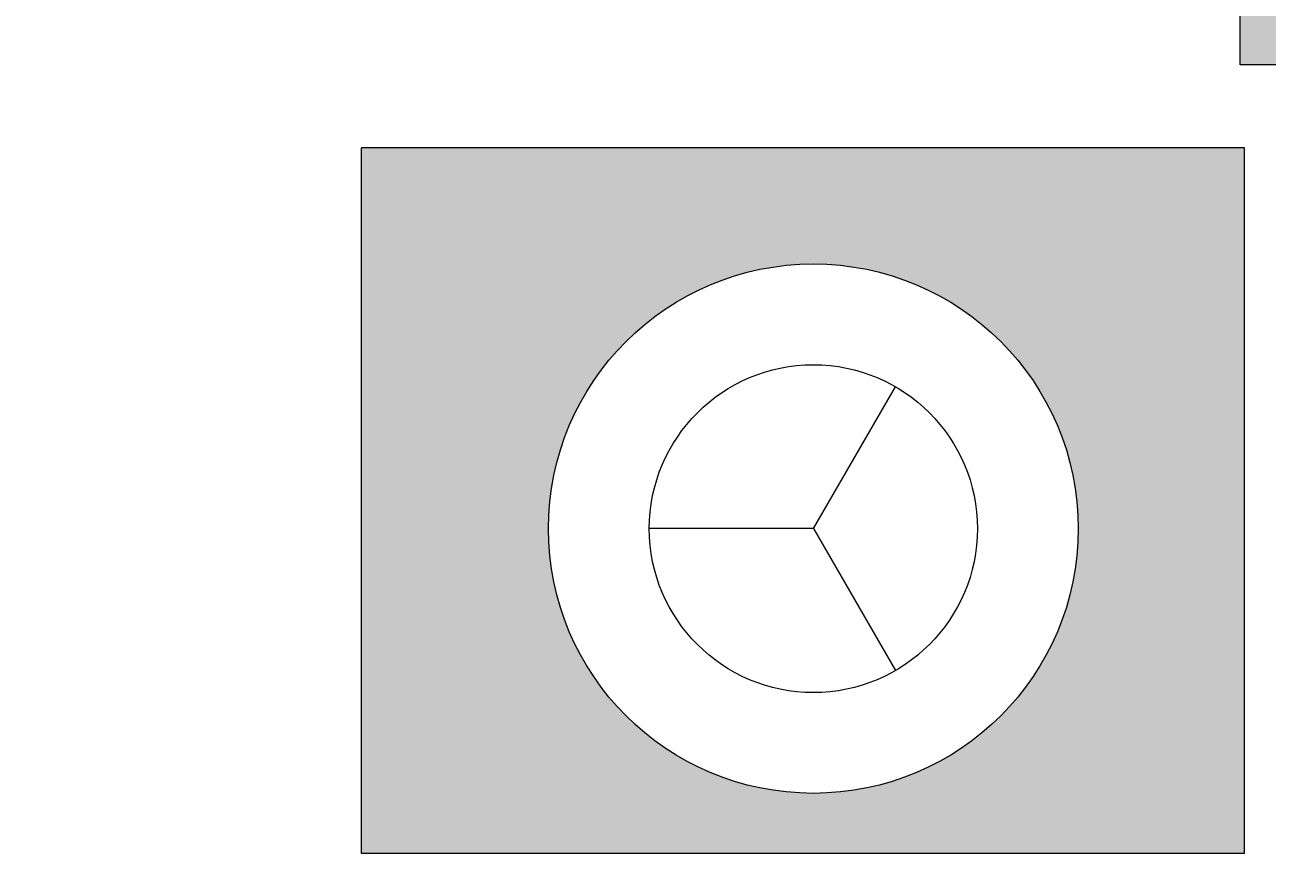
# Model space of a CAD drawing. Units: millimetres. Extents: x 27017497 to 27018854, y 7058029 to 7059154.
# Tile 20 of 91: x 27017651 to 27017679, y 7058144 to 7058163. Entities that reach past the tile are written whole.
import ezdxf

# ---------------------------------------------------------------- set-up
doc = ezdxf.new("R2010")
doc.units = ezdxf.units.MM
doc.layers.add('A-ANNO-DIMS', color=2, linetype='Continuous', lineweight=18)
doc.layers.add('A-FURN', color=8, linetype='Continuous', lineweight=18)
doc.layers.add('A-FURN-PATT', color=177, linetype='Continuous', lineweight=13, true_color=0x293189)
doc.styles.get("Standard").update_dxf_attribs({"font": 'arial.ttf'})
doc.dimstyles.get("Standard").update_dxf_attribs({"dimtxt": 0.18, "dimasz": 0.18, "dimexe": 0.18, "dimexo": 0.0625, "dimgap": 0.09, "dimtad": 0, "dimtih": 1, "dimtoh": 1, "dimdec": 4, "dimzin": 0, "dimdsep": 46, "dimtxsty": 'Standard', "dimcen": 0.09, "dimadec": 0, "dimazin": 0, "dimtfac": 1, "dimtdec": 4, "dimtofl": 0, "dimtmove": 0, "dimatfit": 3, "dimfxl": 1, "dimtolj": 1, "dimtzin": 0, "dimarcsym": 0})

# ---------------------------------------------------------------- blocks, each defined once
blk = doc.blocks.new('CAMMAT')
for p, q in [((0.68, -0.07), (0.68, -0.47)), ((0.68, -0.07), (1.18, -0.07)), ((1.18, -0.07), (1.18, -0.47)), ((0.92416, -0.2541), (0.87771, -0.17366)), ((0.92416, -0.2541), (0.87771, -0.33455)), ((0.92416, -0.2541), (1.01705, -0.2541)), ((0.68, -0.47), (1.18, -0.47)), ((-0.6904, -0.51693), (0.68256, -0.51693)), ((0.68256, -0.51693), (0.68256, -0.76028))]:
    blk.add_line(p, q)
for radius in [0.15, 0.09289]:
    blk.add_circle((0.92416, -0.2541), radius)
blk = doc.blocks.new('*D47')
at = {"layer": 'A-ANNO-DIMS', "color": 0, "lineweight": -2, "transparency": 16777216}
for p, q in [((27017561.166, 7058294.35), (27017561.166, 7058028.6)), ((27018790.606, 7058294.35), (27018790.606, 7058028.6)), ((27017561.346, 7058028.78), (27018175.431, 7058028.78)), ((27018790.426, 7058028.78), (27018176.341, 7058028.78))]:
    blk.add_line(p, q, dxfattribs=at)
at = {"layer": 'A-ANNO-DIMS', "color": 0, "transparency": 16777216}
for points in [[(27017561.346, 7058028.81), (27017561.346, 7058028.75), (27017561.166, 7058028.78)], [(27018790.426, 7058028.81), (27018790.426, 7058028.75), (27018790.606, 7058028.78)]]:
    blk.add_solid(points, dxfattribs=at)
at = {"layer": 'Defpoints', "color": 0, "transparency": 16777216}
for p in [(27017561.166, 7058294.412), (27018790.606, 7058294.412), (27018790.606, 7058028.78)]:
    blk.add_point(p, dxfattribs=at)
at = {"layer": 'A-ANNO-DIMS', "color": 0, "transparency": 16777216, "insert": (27018175.886, 7058028.78), "char_height": 0.18, "attachment_point": 5}
blk.add_mtext('\\A1;1229.4', dxfattribs=at)
blk = doc.blocks.new('*D48')
at = {"layer": 'A-ANNO-DIMS', "color": 0, "lineweight": -2, "transparency": 16777216}
for p, q in [((27018463.498, 7058622.912), (27017497.536, 7058622.912)), ((27017497.716, 7058622.732), (27017497.716, 7058357.753)), ((27017497.716, 7058092.41), (27017497.716, 7058357.389)), ((27018555.129, 7058092.23), (27017497.536, 7058092.23))]:
    blk.add_line(p, q, dxfattribs=at)
at = {"layer": 'A-ANNO-DIMS', "color": 0, "transparency": 16777216}
for points in [[(27017497.686, 7058622.732), (27017497.746, 7058622.732), (27017497.716, 7058622.912)], [(27017497.686, 7058092.41), (27017497.746, 7058092.41), (27017497.716, 7058092.23)]]:
    blk.add_solid(points, dxfattribs=at)
at = {"layer": 'Defpoints', "color": 0, "transparency": 16777216}
for p in [(27018463.561, 7058622.912), (27017497.716, 7058092.23), (27018555.192, 7058092.23)]:
    blk.add_point(p, dxfattribs=at)
at = {"layer": 'A-ANNO-DIMS', "color": 0, "transparency": 16777216, "insert": (27017497.716, 7058357.571), "char_height": 0.18, "attachment_point": 5}
blk.add_mtext('\\A1;530.7', dxfattribs=at)

msp = doc.modelspace()

# ---------------------------------------------------------------- hatches: boundary and pattern name
at = {"layer": 'A-FURN-PATT'}
h = msp.add_hatch(color=256, dxfattribs=at)
h.dxf.hatch_style = 1
h.paths.add_polyline_path([(27017731.53, 7058218.852, 0.414214), (27017729.937, 7058220.445), (27017681.344, 7058220.445, 0.414214), (27017679.751, 7058218.852), (27017679.751, 7058174.658), (27017683.647, 7058174.959), (27017687.23, 7058175.46), (27017689.748, 7058176.196), (27017691.461, 7058177.277), (27017692.628, 7058178.816), (27017693.508, 7058180.922), (27017694.36, 7058183.707), (27017694.963, 7058180.902), (27017695.506, 7058178.662), (27017696.096, 7058176.759), (27017696.84, 7058174.966), (27017697.847, 7058173.059), (27017699.222, 7058170.809), (27017701.073, 7058167.99), (27017703.508, 7058164.376), (27017705.943, 7058167.99), (27017707.794, 7058170.809), (27017709.169, 7058173.059), (27017710.176, 7058174.966), (27017710.92, 7058176.759), (27017711.51, 7058178.662), (27017712.053, 7058180.902), (27017712.656, 7058183.707), (27017713.508, 7058180.922), (27017714.388, 7058178.816), (27017715.555, 7058177.277), (27017717.268, 7058176.196), (27017719.786, 7058175.46), (27017723.369, 7058174.959), (27017728.274, 7058174.58), (27017731.53, 7058174.396)])
h.paths.add_polyline_path([(27017723.369, 7058174.959), (27017719.786, 7058175.46), (27017717.268, 7058176.196), (27017715.555, 7058177.277), (27017714.388, 7058178.816), (27017713.508, 7058180.922), (27017712.656, 7058183.707), (27017712.053, 7058180.902), (27017711.51, 7058178.662), (27017710.92, 7058176.759), (27017710.176, 7058174.966), (27017709.169, 7058173.059), (27017707.794, 7058170.809), (27017705.943, 7058167.99), (27017703.508, 7058164.376), (27017734.763, 7058174.214), (27017728.274, 7058174.58)])
h.paths.add_polyline_path([(27017696.84, 7058174.966), (27017696.096, 7058176.759), (27017695.506, 7058178.662), (27017694.963, 7058180.902), (27017694.36, 7058183.707), (27017693.508, 7058180.922), (27017692.628, 7058178.816), (27017691.461, 7058177.277), (27017689.748, 7058176.196), (27017687.23, 7058175.46), (27017683.647, 7058174.959), (27017679.751, 7058174.658), (27017678.741, 7058174.58), (27017672.253, 7058174.214), (27017703.508, 7058164.376), (27017701.073, 7058167.99), (27017699.222, 7058170.809), (27017697.847, 7058173.059)])
h.paths.add_polyline_path([(27017678.454, 7058172.262), (27017678.454, 7058162.569), (27017733.139, 7058162.569), (27017733.139, 7058173.703), (27017703.508, 7058164.376)])
h.paths.add_polyline_path([(27017730.145, 7058158.291, 0.41419), (27017728.95, 7058159.485), (27017707.491, 7058159.485, 0.414214), (27017706.296, 7058158.29), (27017706.296, 7058148.731, 0.414214), (27017707.491, 7058147.536), (27017728.95, 7058147.536, 0.414237), (27017730.145, 7058148.731)], flags=0)
h.paths.add_polyline_path([(27017731.53, 7058162.569), (27017679.751, 7058162.569), (27017679.751, 7058146.361, 0.414214), (27017681.344, 7058144.768), (27017729.937, 7058144.768, 0.414214), (27017731.53, 7058146.361)])
h.paths.add_polyline_path([(27017703.354, 7058159.485, -0.41419), (27017704.549, 7058158.291), (27017704.549, 7058148.731, -0.414237), (27017703.354, 7058147.536), (27017681.894, 7058147.536, -0.41419), (27017680.699, 7058148.731), (27017680.699, 7058158.29, -0.414237), (27017681.894, 7058159.485)], flags=0)
h.paths.add_polyline_path([(27017707.491, 7058159.485), (27017728.95, 7058159.485, -0.41419), (27017730.145, 7058158.291), (27017730.145, 7058148.731, -0.414237), (27017728.95, 7058147.536), (27017707.491, 7058147.536, -0.414214), (27017706.296, 7058148.731), (27017706.296, 7058158.29, -0.414214)], flags=16)
h.paths.add_polyline_path([(27017704.549, 7058158.291, 0.41419), (27017703.354, 7058159.485), (27017681.894, 7058159.485, 0.414237), (27017680.699, 7058158.29), (27017680.699, 7058148.731, 0.41419), (27017681.894, 7058147.536), (27017703.354, 7058147.536, 0.414237), (27017704.549, 7058148.731)], flags=16)
h.paths.add_polyline_path([(27017752.64, 7058160.7), (27017732.725, 7058160.7), (27017732.725, 7058144.768), (27017752.64, 7058144.768)])
h.paths.add_polyline_path([(27017748.698, 7058152.101, -1), (27017736.749, 7058152.101, -1)], flags=16)
h.paths.add_polyline_path([(27017746.424, 7058152.101, -1), (27017739.024, 7058152.101, -1)], flags=0)
h.paths.add_polyline_path([(27017678.556, 7058160.7), (27017658.641, 7058160.7), (27017658.641, 7058144.768), (27017678.556, 7058144.768)])
h.paths.add_polyline_path([(27017674.806, 7058152.101, -1), (27017662.857, 7058152.101, -1)], flags=16)
h.paths.add_polyline_path([(27017672.531, 7058152.101, -1), (27017665.131, 7058152.101, -1)], flags=0)

# ---------------------------------------------------------------- block references
at = {"layer": 'A-FURN', "xscale": 39.82996475819422, "yscale": 39.82996475819422, "zscale": 39.82996475819422, "rotation": 180}
msp.add_blockref('CAMMAT', (27017705.64, 7058141.98), dxfattribs=at)

# ---------------------------------------------------------------- dimensions: what is measured, and where the dimension line sits
at = {"layer": 'A-ANNO-DIMS'}
dim = msp.add_linear_dim(base=(27017497.716, 7058092.23), p1=(27018463.561, 7058622.912), p2=(27018555.192, 7058092.23), angle=90, dimstyle='Standard', override={"dimdec": 1, "dimlfac": 1, "dimrnd": 0, "dimzin": 0, "dimdsep": 46, "dimlunit": 2}, dxfattribs=at)
dim.commit()
dim.dimension.update_dxf_attribs({"geometry": '*D48', "text_midpoint": (27017497.716, 7058357.571)})
dim = msp.add_linear_dim(base=(27018790.606, 7058028.78), p1=(27017561.166, 7058294.412), p2=(27018790.606, 7058294.412), dimstyle='Standard', override={"dimdec": 1, "dimlfac": 1, "dimrnd": 0, "dimzin": 0, "dimdsep": 46, "dimlunit": 2}, dxfattribs=at)
dim.commit()
dim.dimension.update_dxf_attribs({"geometry": '*D47', "text_midpoint": (27018175.886, 7058028.78)})

doc.saveas('drawing.dxf')
